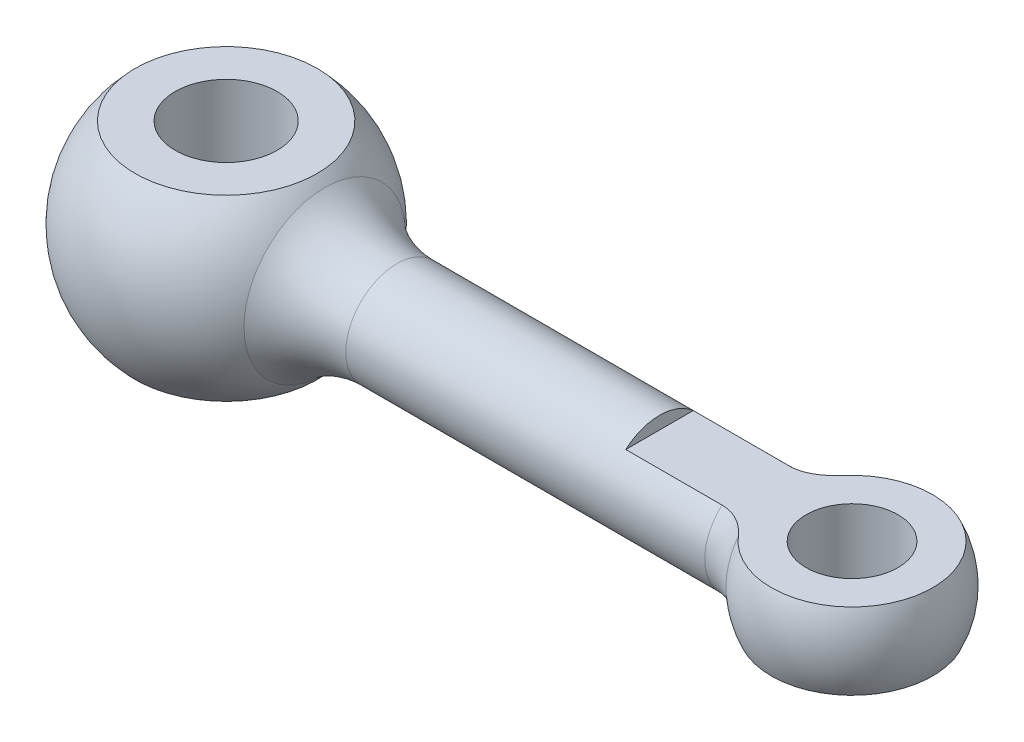
ISO-10303-21;
HEADER;
FILE_DESCRIPTION(('STEP AP214'),'2;1');
FILE_NAME('part.step','',(''),(''),'','','');
FILE_SCHEMA(('AUTOMOTIVE_DESIGN { 1 0 10303 214 1 1 1 1 }'));
ENDSEC;
DATA;
#1=APPLICATION_CONTEXT('core data for automotive mechanical design processes');
#2=APPLICATION_PROTOCOL_DEFINITION('international standard','automotive_design',2000,#1);
#3=PRODUCT_CONTEXT('',#1,'mechanical');
#4=PRODUCT('Part','Part','',(#3));
#5=PRODUCT_RELATED_PRODUCT_CATEGORY('part','',(#4));
#6=PRODUCT_DEFINITION_FORMATION('','',#4);
#7=PRODUCT_DEFINITION_CONTEXT('part definition',#1,'design');
#8=PRODUCT_DEFINITION('design','',#6,#7);
#9=PRODUCT_DEFINITION_SHAPE('','',#8);
#10=(LENGTH_UNIT() NAMED_UNIT(*) SI_UNIT(.MILLI.,.METRE.));
#11=(NAMED_UNIT(*) PLANE_ANGLE_UNIT() SI_UNIT($,.RADIAN.));
#12=(NAMED_UNIT(*) SI_UNIT($,.STERADIAN.) SOLID_ANGLE_UNIT());
#13=UNCERTAINTY_MEASURE_WITH_UNIT(LENGTH_MEASURE(1.E-05),#10,'distance_accuracy_value','');
#14=(GEOMETRIC_REPRESENTATION_CONTEXT(3) GLOBAL_UNCERTAINTY_ASSIGNED_CONTEXT((#13)) GLOBAL_UNIT_ASSIGNED_CONTEXT((#10,
#11,#12)) REPRESENTATION_CONTEXT('',''));
#15=CARTESIAN_POINT('',(0.,0.,0.));
#16=DIRECTION('',(0.,0.,1.));
#17=DIRECTION('',(1.,0.,0.));
#18=AXIS2_PLACEMENT_3D('',#15,#16,#17);
#19=CARTESIAN_POINT('',(-51.35,0.,0.));
#20=DIRECTION('',(-1.,0.,0.));
#21=DIRECTION('',(0.,0.,1.));
#22=AXIS2_PLACEMENT_3D('',#19,#20,#21);
#23=CYLINDRICAL_SURFACE('',#22,10.);
#24=CARTESIAN_POINT('',(-27.8839339326469,0.,0.));
#25=DIRECTION('',(-1.,0.,0.));
#26=DIRECTION('',(0.,0.,1.));
#27=AXIS2_PLACEMENT_3D('',#24,#25,#26);
#28=CIRCLE('',#27,10.);
#29=CARTESIAN_POINT('',(-27.8839339326469,0.,10.));
#30=VERTEX_POINT('',#29);
#31=EDGE_CURVE('E124',#30,#30,#28,.T.);
#32=ORIENTED_EDGE('',*,*,#31,.F.);
#33=EDGE_LOOP('',(#32));
#34=FACE_BOUND('',#33,.T.);
#35=CARTESIAN_POINT('',(23.61,0.,0.));
#36=DIRECTION('',(-1.,0.,0.));
#37=DIRECTION('',(0.,0.,1.));
#38=AXIS2_PLACEMENT_3D('',#35,#36,#37);
#39=CIRCLE('',#38,10.);
#40=CARTESIAN_POINT('',(23.61,-7.5,-6.61437827766148));
#41=VERTEX_POINT('',#40);
#42=CARTESIAN_POINT('',(23.61,-7.5,6.61437827766148));
#43=VERTEX_POINT('',#42);
#44=EDGE_CURVE('E106',#41,#43,#39,.T.);
#45=ORIENTED_EDGE('',*,*,#44,.T.);
#46=DIRECTION('',(1.,0.,0.));
#47=VECTOR('',#46,1.);
#48=CARTESIAN_POINT('',(23.61,-7.5,6.61437827766148));
#49=LINE('',#48,#47);
#50=CARTESIAN_POINT('',(42.4754139118231,-7.5,6.61437827766148));
#51=VERTEX_POINT('',#50);
#52=EDGE_CURVE('E99',#43,#51,#49,.T.);
#53=ORIENTED_EDGE('',*,*,#52,.T.);
#54=CARTESIAN_POINT('',(42.4754139118231,0.,0.));
#55=DIRECTION('',(1.,0.,0.));
#56=DIRECTION('',(0.,0.,-1.));
#57=AXIS2_PLACEMENT_3D('',#54,#55,#56);
#58=CIRCLE('',#57,10.);
#59=CARTESIAN_POINT('',(42.4754139118231,7.5,6.61437827766148));
#60=VERTEX_POINT('',#59);
#61=EDGE_CURVE('E104',#51,#60,#58,.F.);
#62=ORIENTED_EDGE('',*,*,#61,.T.);
#63=DIRECTION('',(1.,0.,0.));
#64=VECTOR('',#63,1.);
#65=CARTESIAN_POINT('',(23.61,7.5,6.61437827766148));
#66=LINE('',#65,#64);
#67=CARTESIAN_POINT('',(23.61,7.5,6.61437827766148));
#68=VERTEX_POINT('',#67);
#69=EDGE_CURVE('E320',#68,#60,#66,.T.);
#70=ORIENTED_EDGE('',*,*,#69,.F.);
#71=CARTESIAN_POINT('',(23.61,0.,0.));
#72=DIRECTION('',(1.,0.,0.));
#73=DIRECTION('',(0.,0.,-1.));
#74=AXIS2_PLACEMENT_3D('',#71,#72,#73);
#75=CIRCLE('',#74,10.);
#76=CARTESIAN_POINT('',(23.61,7.5,-6.61437827766148));
#77=VERTEX_POINT('',#76);
#78=EDGE_CURVE('E314',#77,#68,#75,.T.);
#79=ORIENTED_EDGE('',*,*,#78,.F.);
#80=DIRECTION('',(-1.,0.,0.));
#81=VECTOR('',#80,1.);
#82=CARTESIAN_POINT('',(52.35,7.5,-6.61437827766148));
#83=LINE('',#82,#81);
#84=CARTESIAN_POINT('',(42.4754139118231,7.5,-6.61437827766148));
#85=VERTEX_POINT('',#84);
#86=EDGE_CURVE('E173',#85,#77,#83,.T.);
#87=ORIENTED_EDGE('',*,*,#86,.F.);
#88=CARTESIAN_POINT('',(42.4754139118231,0.,0.));
#89=DIRECTION('',(1.,0.,0.));
#90=DIRECTION('',(0.,0.,-1.));
#91=AXIS2_PLACEMENT_3D('',#88,#89,#90);
#92=CIRCLE('',#91,10.);
#93=CARTESIAN_POINT('',(42.4754139118231,-7.5,-6.61437827766148));
#94=VERTEX_POINT('',#93);
#95=EDGE_CURVE('E120',#85,#94,#92,.F.);
#96=ORIENTED_EDGE('',*,*,#95,.T.);
#97=DIRECTION('',(-1.,0.,0.));
#98=VECTOR('',#97,1.);
#99=CARTESIAN_POINT('',(52.35,-7.5,-6.61437827766148));
#100=LINE('',#99,#98);
#101=EDGE_CURVE('E171',#94,#41,#100,.T.);
#102=ORIENTED_EDGE('',*,*,#101,.T.);
#103=EDGE_LOOP('',(#45,#53,#62,#70,#79,#87,#96,#102));
#104=FACE_BOUND('',#103,.T.);
#105=ADVANCED_FACE('F41',(#34,#104),#23,.T.);
#106=CARTESIAN_POINT('',(-61.35,0.,0.));
#107=DIRECTION('',(0.,-1.,0.));
#108=DIRECTION('',(-1.,0.,0.));
#109=AXIS2_PLACEMENT_3D('',#106,#107,#108);
#110=SPHERICAL_SURFACE('',#109,25.);
#111=CARTESIAN_POINT('',(-61.35,17.5,0.));
#112=DIRECTION('',(0.,-1.,0.));
#113=DIRECTION('',(0.,0.,-1.));
#114=AXIS2_PLACEMENT_3D('',#111,#112,#113);
#115=CIRCLE('',#114,17.8535710713572);
#116=CARTESIAN_POINT('',(-61.35,17.5,-17.8535710713572));
#117=VERTEX_POINT('',#116);
#118=EDGE_CURVE('E194',#117,#117,#115,.T.);
#119=ORIENTED_EDGE('',*,*,#118,.T.);
#120=EDGE_LOOP('',(#119));
#121=FACE_BOUND('',#120,.T.);
#122=CARTESIAN_POINT('',(-42.0098077527709,0.,0.));
#123=DIRECTION('',(1.,0.,0.));
#124=DIRECTION('',(0.,0.,-1.));
#125=AXIS2_PLACEMENT_3D('',#122,#123,#124);
#126=CIRCLE('',#125,15.8416212503714);
#127=CARTESIAN_POINT('',(-42.0098077527709,0.,-15.8416212503714));
#128=VERTEX_POINT('',#127);
#129=EDGE_CURVE('E130',#128,#128,#126,.T.);
#130=ORIENTED_EDGE('',*,*,#129,.F.);
#131=EDGE_LOOP('',(#130));
#132=FACE_BOUND('',#131,.T.);
#133=CARTESIAN_POINT('',(-61.35,-17.5,0.));
#134=DIRECTION('',(0.,-1.,0.));
#135=DIRECTION('',(0.,0.,-1.));
#136=AXIS2_PLACEMENT_3D('',#133,#134,#135);
#137=CIRCLE('',#136,17.8535710713571);
#138=CARTESIAN_POINT('',(-61.35,-17.5,-17.8535710713571));
#139=VERTEX_POINT('',#138);
#140=EDGE_CURVE('E195',#139,#139,#137,.T.);
#141=ORIENTED_EDGE('',*,*,#140,.F.);
#142=EDGE_LOOP('',(#141));
#143=FACE_BOUND('',#142,.T.);
#144=ADVANCED_FACE('F203',(#121,#132,#143),#110,.T.);
#145=CARTESIAN_POINT('',(0.,17.5,0.));
#146=DIRECTION('',(0.,-1.,0.));
#147=DIRECTION('',(0.,0.,-1.));
#148=AXIS2_PLACEMENT_3D('',#145,#146,#147);
#149=PLANE('',#148);
#150=ORIENTED_EDGE('',*,*,#118,.F.);
#151=EDGE_LOOP('',(#150));
#152=FACE_BOUND('',#151,.T.);
#153=CARTESIAN_POINT('',(-61.35,17.5,0.));
#154=DIRECTION('',(0.,-1.,0.));
#155=DIRECTION('',(0.,0.,-1.));
#156=AXIS2_PLACEMENT_3D('',#153,#154,#155);
#157=CIRCLE('',#156,10.);
#158=CARTESIAN_POINT('',(-61.35,17.5,-10.));
#159=VERTEX_POINT('',#158);
#160=EDGE_CURVE('E179',#159,#159,#157,.T.);
#161=ORIENTED_EDGE('',*,*,#160,.T.);
#162=EDGE_LOOP('',(#161));
#163=FACE_BOUND('',#162,.T.);
#164=ADVANCED_FACE('F204',(#152,#163),#149,.F.);
#165=CARTESIAN_POINT('',(0.,-17.5,0.));
#166=DIRECTION('',(0.,-1.,0.));
#167=DIRECTION('',(0.,0.,-1.));
#168=AXIS2_PLACEMENT_3D('',#165,#166,#167);
#169=PLANE('',#168);
#170=ORIENTED_EDGE('',*,*,#140,.T.);
#171=EDGE_LOOP('',(#170));
#172=FACE_BOUND('',#171,.T.);
#173=CARTESIAN_POINT('',(-61.35,-17.5,0.));
#174=DIRECTION('',(0.,-1.,0.));
#175=DIRECTION('',(0.,0.,-1.));
#176=AXIS2_PLACEMENT_3D('',#173,#174,#175);
#177=CIRCLE('',#176,10.);
#178=CARTESIAN_POINT('',(-61.35,-17.5,-10.));
#179=VERTEX_POINT('',#178);
#180=EDGE_CURVE('E183',#179,#179,#177,.T.);
#181=ORIENTED_EDGE('',*,*,#180,.F.);
#182=EDGE_LOOP('',(#181));
#183=FACE_BOUND('',#182,.T.);
#184=ADVANCED_FACE('F209',(#172,#183),#169,.T.);
#185=CARTESIAN_POINT('',(-61.35,-17.5,0.));
#186=DIRECTION('',(0.,-1.,0.));
#187=DIRECTION('',(0.,0.,-1.));
#188=AXIS2_PLACEMENT_3D('',#185,#186,#187);
#189=CYLINDRICAL_SURFACE('',#188,10.);
#190=ORIENTED_EDGE('',*,*,#160,.F.);
#191=EDGE_LOOP('',(#190));
#192=FACE_BOUND('',#191,.T.);
#193=ORIENTED_EDGE('',*,*,#180,.T.);
#194=EDGE_LOOP('',(#193));
#195=FACE_BOUND('',#194,.T.);
#196=ADVANCED_FACE('F157',(#192,#195),#189,.F.);
#197=CARTESIAN_POINT('',(-27.8839339326469,0.,0.));
#198=DIRECTION('',(-1.,0.,0.));
#199=DIRECTION('',(0.,0.,1.));
#200=AXIS2_PLACEMENT_3D('',#197,#198,#199);
#201=TOROIDAL_SURFACE('',#200,30.,20.);
#202=ORIENTED_EDGE('',*,*,#31,.T.);
#203=EDGE_LOOP('',(#202));
#204=FACE_BOUND('',#203,.T.);
#205=ORIENTED_EDGE('',*,*,#129,.T.);
#206=EDGE_LOOP('',(#205));
#207=FACE_BOUND('',#206,.T.);
#208=ADVANCED_FACE('F156',(#204,#207),#201,.F.);
#209=CARTESIAN_POINT('',(0.,-7.5,0.));
#210=DIRECTION('',(0.,-1.,0.));
#211=DIRECTION('',(0.,0.,-1.));
#212=AXIS2_PLACEMENT_3D('',#209,#210,#211);
#213=PLANE('',#212);
#214=CARTESIAN_POINT('',(61.35,-7.5,0.));
#215=DIRECTION('',(0.,1.,0.));
#216=DIRECTION('',(0.,0.,1.));
#217=AXIS2_PLACEMENT_3D('',#214,#215,#216);
#218=CIRCLE('',#217,8.99999999999999);
#219=CARTESIAN_POINT('',(61.35,-7.5,8.99999999999999));
#220=VERTEX_POINT('',#219);
#221=EDGE_CURVE('E316',#220,#220,#218,.T.);
#222=ORIENTED_EDGE('',*,*,#221,.T.);
#223=EDGE_LOOP('',(#222));
#224=FACE_BOUND('',#223,.T.);
#225=ORIENTED_EDGE('',*,*,#101,.F.);
#226=CARTESIAN_POINT('',(42.4754139118231,-7.5,-6.61437827766148));
#227=CARTESIAN_POINT('',(42.5925058437068,-7.5,-6.61436536840376));
#228=CARTESIAN_POINT('',(42.709592666835,-7.5,-6.61748719737454));
#229=CARTESIAN_POINT('',(42.943420180467,-7.5,-6.62990378667274));
#230=CARTESIAN_POINT('',(43.0601609240622,-7.5,-6.63919754508578));
#231=CARTESIAN_POINT('',(43.2927711788786,-7.5,-6.66383741850007));
#232=CARTESIAN_POINT('',(43.4086419464541,-7.5,-6.67917167617335));
#233=CARTESIAN_POINT('',(43.6394463945103,-7.5,-6.71570865496497));
#234=CARTESIAN_POINT('',(43.7543800475365,-7.5,-6.73691154738473));
#235=CARTESIAN_POINT('',(44.0942923347153,-7.5,-6.8083483773029));
#236=CARTESIAN_POINT('',(44.31759618933,-7.5,-6.86676285088429));
#237=CARTESIAN_POINT('',(44.7580368822529,-7.5,-7.00348482977181));
#238=CARTESIAN_POINT('',(44.9751708570763,-7.5,-7.08180140938989));
#239=CARTESIAN_POINT('',(45.4004039772594,-7.5,-7.25528780700288));
#240=CARTESIAN_POINT('',(45.6085642250108,-7.5,-7.35030873359448));
#241=CARTESIAN_POINT('',(46.0171868598969,-7.5,-7.55555009507107));
#242=CARTESIAN_POINT('',(46.2176497745284,-7.5,-7.66576948602297));
#243=CARTESIAN_POINT('',(46.6116678805253,-7.5,-7.90024828949096));
#244=CARTESIAN_POINT('',(46.805178397922,-7.5,-8.02458245539592));
#245=CARTESIAN_POINT('',(47.183933702627,-7.5,-8.2852665806018));
#246=CARTESIAN_POINT('',(47.3691776437801,-7.5,-8.4216177657177));
#247=CARTESIAN_POINT('',(47.7140547360645,-7.5,-8.69162305433913));
#248=CARTESIAN_POINT('',(47.8744506651147,-7.5,-8.82430664399124));
#249=CARTESIAN_POINT('',(48.1882219262494,-7.5,-9.09772037514378));
#250=CARTESIAN_POINT('',(48.3415973390705,-7.5,-9.23845042406732));
#251=CARTESIAN_POINT('',(48.6397765110251,-7.5,-9.52594059289856));
#252=CARTESIAN_POINT('',(48.784647872087,-7.5,-9.67263070570517));
#253=CARTESIAN_POINT('',(49.0671983230259,-7.5,-9.97273469005625));
#254=CARTESIAN_POINT('',(49.2048786894703,-7.5,-10.1261473592384));
#255=CARTESIAN_POINT('',(49.3388997620693,-7.5,-10.2826782053306));
#256=B_SPLINE_CURVE_WITH_KNOTS('',3,(#226,#227,#228,#229,#230,#231,#232,#233,#234,#235,#236,
#237,#238,#239,#240,#241,#242,#243,#244,#245,#246,#247,#248,#249,#250,#251,#252,#253,#254,#255),
.UNSPECIFIED.,.F.,.F.,(4,2,2,2,2,2,2,2,2,2,2,2,2,2,4),(0.,0.35122561716206,0.702394232375438,
1.05287692143297,1.40336984191939,2.09469953424882,2.78634500382609,3.47211222843016,
4.15783237335545,4.84737037465873,5.53697879496275,6.16118840793274,6.78539084063059,
7.40366187726206,8.02182278084558),.UNSPECIFIED.);
#257=CARTESIAN_POINT('',(49.3388997620693,-7.5,-10.2826782053306));
#258=VERTEX_POINT('',#257);
#259=EDGE_CURVE('E54',#94,#258,#256,.T.);
#260=ORIENTED_EDGE('',*,*,#259,.T.);
#261=CARTESIAN_POINT('',(61.35,-7.5,0.));
#262=DIRECTION('',(0.,1.,0.));
#263=DIRECTION('',(0.,0.,1.));
#264=AXIS2_PLACEMENT_3D('',#261,#262,#263);
#265=CIRCLE('',#264,15.8113883008419);
#266=CARTESIAN_POINT('',(49.3388997620693,-7.5,10.2826782053306));
#267=VERTEX_POINT('',#266);
#268=EDGE_CURVE('E112',#267,#258,#265,.T.);
#269=ORIENTED_EDGE('',*,*,#268,.F.);
#270=CARTESIAN_POINT('',(49.3388997620693,-7.49999999999999,10.2826782053306));
#271=CARTESIAN_POINT('',(49.2386622528365,-7.5,10.1655963271284));
#272=CARTESIAN_POINT('',(49.1363838937134,-7.5,10.0502756668184));
#273=CARTESIAN_POINT('',(48.9277914432878,-7.5,9.82333345458339));
#274=CARTESIAN_POINT('',(48.8214771402463,-7.5,9.7117120973132));
#275=CARTESIAN_POINT('',(48.4962524179336,-7.5,9.38236325800093));
#276=CARTESIAN_POINT('',(48.2713501510137,-7.5,9.17049044639498));
#277=CARTESIAN_POINT('',(47.8021904176805,-7.5,8.76101162314677));
#278=CARTESIAN_POINT('',(47.5576723400671,-7.5,8.56370314078696));
#279=CARTESIAN_POINT('',(47.0532809530385,-7.5,8.19025013825436));
#280=CARTESIAN_POINT('',(46.7934182836623,-7.5,8.01409120406649));
#281=CARTESIAN_POINT('',(46.141526951436,-7.5,7.61469794499551));
#282=CARTESIAN_POINT('',(45.7412559008822,-7.5,7.40440682467836));
#283=CARTESIAN_POINT('',(45.1216394865351,-7.5,7.1387213780044));
#284=CARTESIAN_POINT('',(44.9126820764037,-7.5,7.05865055914743));
#285=CARTESIAN_POINT('',(44.4886569182098,-7.5,6.91668412867678));
#286=CARTESIAN_POINT('',(44.2735918511918,-7.5,6.85478067346105));
#287=CARTESIAN_POINT('',(43.9272450946036,-7.5,6.77224834601358));
#288=CARTESIAN_POINT('',(43.7974926251357,-7.5,6.74507533763384));
#289=CARTESIAN_POINT('',(43.5366662471307,-7.5,6.69817157720569));
#290=CARTESIAN_POINT('',(43.4055926564705,-7.5,6.67843907679756));
#291=CARTESIAN_POINT('',(43.141613011337,-7.5,6.64659622209488));
#292=CARTESIAN_POINT('',(43.0087005557848,-7.5,6.63453880868027));
#293=CARTESIAN_POINT('',(42.7423331317098,-7.5,6.61841717549713));
#294=CARTESIAN_POINT('',(42.6088779462773,-7.5,6.6143565493105));
#295=CARTESIAN_POINT('',(42.4754139118231,-7.5,6.61437827766148));
#296=B_SPLINE_CURVE_WITH_KNOTS('',3,(#270,#271,#272,#273,#274,#275,#276,#277,#278,#279,#280,
#281,#282,#283,#284,#285,#286,#287,#288,#289,#290,#291,#292,#293,#294,#295),.UNSPECIFIED.,.F.,
.F.,(4,2,2,2,2,2,2,2,2,2,2,2,4),(0.,0.462340238289144,0.924704766101818,1.85076998031453,
2.79230848880958,3.73320162509837,5.08415601680602,5.75484149597022,6.425236985059,
6.8227540340631,7.22017761679553,7.62031364471571,8.02062944405244),.UNSPECIFIED.);
#297=EDGE_CURVE('E111',#267,#51,#296,.T.);
#298=ORIENTED_EDGE('',*,*,#297,.T.);
#299=ORIENTED_EDGE('',*,*,#52,.F.);
#300=DIRECTION('',(0.,0.,1.));
#301=VECTOR('',#300,1.);
#302=CARTESIAN_POINT('',(23.61,-7.5,-6.61437827766147));
#303=LINE('',#302,#301);
#304=EDGE_CURVE('E61',#41,#43,#303,.T.);
#305=ORIENTED_EDGE('',*,*,#304,.F.);
#306=EDGE_LOOP('',(#225,#260,#269,#298,#299,#305));
#307=FACE_BOUND('',#306,.T.);
#308=ADVANCED_FACE('F115',(#224,#307),#213,.T.);
#309=CARTESIAN_POINT('',(61.35,0.,0.));
#310=DIRECTION('',(0.,1.,0.));
#311=DIRECTION('',(1.,0.,0.));
#312=AXIS2_PLACEMENT_3D('',#309,#310,#311);
#313=SPHERICAL_SURFACE('',#312,17.5);
#314=ORIENTED_EDGE('',*,*,#268,.T.);
#315=CARTESIAN_POINT('',(49.3388997620693,0.,0.));
#316=DIRECTION('',(1.,0.,0.));
#317=DIRECTION('',(0.,0.,-1.));
#318=AXIS2_PLACEMENT_3D('',#315,#316,#317);
#319=CIRCLE('',#318,12.7272727272727);
#320=CARTESIAN_POINT('',(49.3388997620693,7.5,-10.2826782053306));
#321=VERTEX_POINT('',#320);
#322=EDGE_CURVE('E166',#258,#321,#319,.T.);
#323=ORIENTED_EDGE('',*,*,#322,.T.);
#324=CARTESIAN_POINT('',(61.35,7.5,0.));
#325=DIRECTION('',(0.,1.,0.));
#326=DIRECTION('',(0.,0.,1.));
#327=AXIS2_PLACEMENT_3D('',#324,#325,#326);
#328=CIRCLE('',#327,15.8113883008419);
#329=CARTESIAN_POINT('',(49.3388997620693,7.5,10.2826782053306));
#330=VERTEX_POINT('',#329);
#331=EDGE_CURVE('E181',#330,#321,#328,.T.);
#332=ORIENTED_EDGE('',*,*,#331,.F.);
#333=CARTESIAN_POINT('',(49.3388997620693,0.,0.));
#334=DIRECTION('',(1.,0.,0.));
#335=DIRECTION('',(0.,0.,-1.));
#336=AXIS2_PLACEMENT_3D('',#333,#334,#335);
#337=CIRCLE('',#336,12.7272727272727);
#338=EDGE_CURVE('E125',#330,#267,#337,.T.);
#339=ORIENTED_EDGE('',*,*,#338,.T.);
#340=EDGE_LOOP('',(#314,#323,#332,#339));
#341=FACE_BOUND('',#340,.T.);
#342=ADVANCED_FACE('F148',(#341),#313,.T.);
#343=CARTESIAN_POINT('',(0.,7.5,0.));
#344=DIRECTION('',(0.,1.,0.));
#345=DIRECTION('',(0.,0.,1.));
#346=AXIS2_PLACEMENT_3D('',#343,#344,#345);
#347=PLANE('',#346);
#348=CARTESIAN_POINT('',(61.35,7.5,0.));
#349=DIRECTION('',(0.,1.,0.));
#350=DIRECTION('',(0.,0.,1.));
#351=AXIS2_PLACEMENT_3D('',#348,#349,#350);
#352=CIRCLE('',#351,8.99999999999999);
#353=CARTESIAN_POINT('',(61.35,7.5,8.99999999999999));
#354=VERTEX_POINT('',#353);
#355=EDGE_CURVE('E187',#354,#354,#352,.T.);
#356=ORIENTED_EDGE('',*,*,#355,.F.);
#357=EDGE_LOOP('',(#356));
#358=FACE_BOUND('',#357,.T.);
#359=CARTESIAN_POINT('',(49.3388997620693,7.49999999999999,-10.2826782053306));
#360=CARTESIAN_POINT('',(49.2386622528365,7.5,-10.1655963271284));
#361=CARTESIAN_POINT('',(49.1363838937134,7.5,-10.0502756668184));
#362=CARTESIAN_POINT('',(48.9277914432878,7.5,-9.82333345458339));
#363=CARTESIAN_POINT('',(48.8214771402463,7.5,-9.7117120973132));
#364=CARTESIAN_POINT('',(48.4962524179336,7.5,-9.38236325800093));
#365=CARTESIAN_POINT('',(48.2713501510137,7.5,-9.17049044639498));
#366=CARTESIAN_POINT('',(47.8021904176805,7.5,-8.76101162314677));
#367=CARTESIAN_POINT('',(47.5576723400671,7.5,-8.56370314078696));
#368=CARTESIAN_POINT('',(47.0532809530385,7.5,-8.19025013825436));
#369=CARTESIAN_POINT('',(46.7934182836623,7.5,-8.01409120406649));
#370=CARTESIAN_POINT('',(46.141526951436,7.5,-7.61469794499551));
#371=CARTESIAN_POINT('',(45.7412559008822,7.5,-7.40440682467836));
#372=CARTESIAN_POINT('',(45.121639486535,7.5,-7.1387213780044));
#373=CARTESIAN_POINT('',(44.9126820764037,7.5,-7.05865055914743));
#374=CARTESIAN_POINT('',(44.4886569182098,7.5,-6.91668412867678));
#375=CARTESIAN_POINT('',(44.2735918511918,7.5,-6.85478067346105));
#376=CARTESIAN_POINT('',(43.9272450946036,7.5,-6.77224834601358));
#377=CARTESIAN_POINT('',(43.7974926251357,7.5,-6.74507533763384));
#378=CARTESIAN_POINT('',(43.5366662471307,7.5,-6.69817157720568));
#379=CARTESIAN_POINT('',(43.4055926564705,7.5,-6.67843907679756));
#380=CARTESIAN_POINT('',(43.141613011337,7.5,-6.64659622209488));
#381=CARTESIAN_POINT('',(43.0087005557848,7.5,-6.63453880868027));
#382=CARTESIAN_POINT('',(42.7423331317098,7.5,-6.61841717549713));
#383=CARTESIAN_POINT('',(42.6088779462773,7.5,-6.6143565493105));
#384=CARTESIAN_POINT('',(42.4754139118231,7.5,-6.61437827766148));
#385=B_SPLINE_CURVE_WITH_KNOTS('',3,(#359,#360,#361,#362,#363,#364,#365,#366,#367,#368,#369,
#370,#371,#372,#373,#374,#375,#376,#377,#378,#379,#380,#381,#382,#383,#384),.UNSPECIFIED.,.F.,
.F.,(4,2,2,2,2,2,2,2,2,2,2,2,4),(0.,0.462340238289147,0.92470476610182,1.85076998031453,
2.79230848880958,3.73320162509837,5.08415601680602,5.75484149597024,6.42523698505901,
6.82275403406312,7.22017761679554,7.62031364471571,8.02062944405244),.UNSPECIFIED.);
#386=EDGE_CURVE('E11',#321,#85,#385,.T.);
#387=ORIENTED_EDGE('',*,*,#386,.T.);
#388=ORIENTED_EDGE('',*,*,#86,.T.);
#389=DIRECTION('',(0.,0.,1.));
#390=VECTOR('',#389,1.);
#391=CARTESIAN_POINT('',(23.61,7.5,-6.61437827766147));
#392=LINE('',#391,#390);
#393=EDGE_CURVE('E69',#77,#68,#392,.T.);
#394=ORIENTED_EDGE('',*,*,#393,.T.);
#395=ORIENTED_EDGE('',*,*,#69,.T.);
#396=CARTESIAN_POINT('',(42.4754139118231,7.5,6.61437827766148));
#397=CARTESIAN_POINT('',(42.5925058437068,7.5,6.61436536840376));
#398=CARTESIAN_POINT('',(42.709592666835,7.5,6.61748719737454));
#399=CARTESIAN_POINT('',(42.943420180467,7.5,6.62990378667274));
#400=CARTESIAN_POINT('',(43.0601609240622,7.5,6.63919754508578));
#401=CARTESIAN_POINT('',(43.2927711788786,7.5,6.66383741850007));
#402=CARTESIAN_POINT('',(43.4086419464541,7.5,6.67917167617335));
#403=CARTESIAN_POINT('',(43.6394463945103,7.5,6.71570865496497));
#404=CARTESIAN_POINT('',(43.7543800475365,7.5,6.73691154738473));
#405=CARTESIAN_POINT('',(44.0942923347153,7.5,6.8083483773029));
#406=CARTESIAN_POINT('',(44.31759618933,7.5,6.86676285088429));
#407=CARTESIAN_POINT('',(44.7580368822529,7.5,7.00348482977181));
#408=CARTESIAN_POINT('',(44.9751708570763,7.5,7.08180140938989));
#409=CARTESIAN_POINT('',(45.4004039772594,7.5,7.25528780700288));
#410=CARTESIAN_POINT('',(45.6085642250108,7.5,7.35030873359449));
#411=CARTESIAN_POINT('',(46.0171868598969,7.5,7.55555009507107));
#412=CARTESIAN_POINT('',(46.2176497745284,7.5,7.66576948602297));
#413=CARTESIAN_POINT('',(46.6116678805253,7.5,7.90024828949096));
#414=CARTESIAN_POINT('',(46.8051783979221,7.5,8.02458245539592));
#415=CARTESIAN_POINT('',(47.183933702627,7.5,8.2852665806018));
#416=CARTESIAN_POINT('',(47.3691776437801,7.5,8.4216177657177));
#417=CARTESIAN_POINT('',(47.7140547360645,7.5,8.69162305433913));
#418=CARTESIAN_POINT('',(47.8744506651147,7.5,8.82430664399124));
#419=CARTESIAN_POINT('',(48.1882219262494,7.5,9.09772037514378));
#420=CARTESIAN_POINT('',(48.3415973390705,7.5,9.23845042406732));
#421=CARTESIAN_POINT('',(48.6397765110251,7.5,9.52594059289856));
#422=CARTESIAN_POINT('',(48.784647872087,7.5,9.67263070570517));
#423=CARTESIAN_POINT('',(49.0671983230259,7.5,9.97273469005625));
#424=CARTESIAN_POINT('',(49.2048786894703,7.5,10.1261473592384));
#425=CARTESIAN_POINT('',(49.3388997620693,7.5,10.2826782053306));
#426=B_SPLINE_CURVE_WITH_KNOTS('',3,(#396,#397,#398,#399,#400,#401,#402,#403,#404,#405,#406,
#407,#408,#409,#410,#411,#412,#413,#414,#415,#416,#417,#418,#419,#420,#421,#422,#423,#424,#425),
.UNSPECIFIED.,.F.,.F.,(4,2,2,2,2,2,2,2,2,2,2,2,2,2,4),(0.,0.35122561716206,0.702394232375438,
1.05287692143298,1.40336984191939,2.09469953424881,2.78634500382609,3.47211222843016,
4.15783237335545,4.84737037465874,5.53697879496275,6.16118840793274,6.78539084063059,
7.40366187726206,8.02182278084558),.UNSPECIFIED.);
#427=EDGE_CURVE('E117',#60,#330,#426,.T.);
#428=ORIENTED_EDGE('',*,*,#427,.T.);
#429=ORIENTED_EDGE('',*,*,#331,.T.);
#430=EDGE_LOOP('',(#387,#388,#394,#395,#428,#429));
#431=FACE_BOUND('',#430,.T.);
#432=ADVANCED_FACE('F141',(#358,#431),#347,.T.);
#433=CARTESIAN_POINT('',(61.35,7.5,0.));
#434=DIRECTION('',(0.,1.,0.));
#435=DIRECTION('',(0.,0.,1.));
#436=AXIS2_PLACEMENT_3D('',#433,#434,#435);
#437=CYLINDRICAL_SURFACE('',#436,8.99999999999999);
#438=ORIENTED_EDGE('',*,*,#355,.T.);
#439=EDGE_LOOP('',(#438));
#440=FACE_BOUND('',#439,.T.);
#441=ORIENTED_EDGE('',*,*,#221,.F.);
#442=EDGE_LOOP('',(#441));
#443=FACE_BOUND('',#442,.T.);
#444=ADVANCED_FACE('F147',(#440,#443),#437,.F.);
#445=CARTESIAN_POINT('',(42.4754139118231,0.,0.));
#446=DIRECTION('',(1.,0.,0.));
#447=DIRECTION('',(0.,0.,-1.));
#448=AXIS2_PLACEMENT_3D('',#445,#446,#447);
#449=TOROIDAL_SURFACE('',#448,20.,10.);
#450=ORIENTED_EDGE('',*,*,#297,.F.);
#451=ORIENTED_EDGE('',*,*,#338,.F.);
#452=ORIENTED_EDGE('',*,*,#427,.F.);
#453=ORIENTED_EDGE('',*,*,#61,.F.);
#454=EDGE_LOOP('',(#450,#451,#452,#453));
#455=FACE_BOUND('',#454,.T.);
#456=ADVANCED_FACE('F122',(#455),#449,.F.);
#457=CARTESIAN_POINT('',(42.4754139118231,0.,0.));
#458=DIRECTION('',(1.,0.,0.));
#459=DIRECTION('',(0.,0.,-1.));
#460=AXIS2_PLACEMENT_3D('',#457,#458,#459);
#461=TOROIDAL_SURFACE('',#460,20.,10.);
#462=ORIENTED_EDGE('',*,*,#386,.F.);
#463=ORIENTED_EDGE('',*,*,#322,.F.);
#464=ORIENTED_EDGE('',*,*,#259,.F.);
#465=ORIENTED_EDGE('',*,*,#95,.F.);
#466=EDGE_LOOP('',(#462,#463,#464,#465));
#467=FACE_BOUND('',#466,.T.);
#468=ADVANCED_FACE('F43',(#467),#461,.F.);
#469=CARTESIAN_POINT('',(23.61,17.501,-6.61437827766147));
#470=DIRECTION('',(1.,0.,0.));
#471=DIRECTION('',(0.,0.,-1.));
#472=AXIS2_PLACEMENT_3D('',#469,#470,#471);
#473=PLANE('',#472);
#474=ORIENTED_EDGE('',*,*,#78,.T.);
#475=ORIENTED_EDGE('',*,*,#393,.F.);
#476=EDGE_LOOP('',(#474,#475));
#477=FACE_BOUND('',#476,.T.);
#478=ADVANCED_FACE('F294',(#477),#473,.T.);
#479=CARTESIAN_POINT('',(23.61,-17.501,-6.61437827766147));
#480=DIRECTION('',(-1.,0.,0.));
#481=DIRECTION('',(0.,0.,1.));
#482=AXIS2_PLACEMENT_3D('',#479,#480,#481);
#483=PLANE('',#482);
#484=ORIENTED_EDGE('',*,*,#304,.T.);
#485=ORIENTED_EDGE('',*,*,#44,.F.);
#486=EDGE_LOOP('',(#484,#485));
#487=FACE_BOUND('',#486,.T.);
#488=ADVANCED_FACE('F297',(#487),#483,.F.);
#489=CLOSED_SHELL('',(#105,#144,#164,#184,#196,#208,#308,#342,#432,#444,#456,#468,#478,#488));
#490=MANIFOLD_SOLID_BREP('B2',#489);
#491=ADVANCED_BREP_SHAPE_REPRESENTATION('',(#18,#490),#14);
#492=SHAPE_DEFINITION_REPRESENTATION(#9,#491);
ENDSEC;
END-ISO-10303-21;
